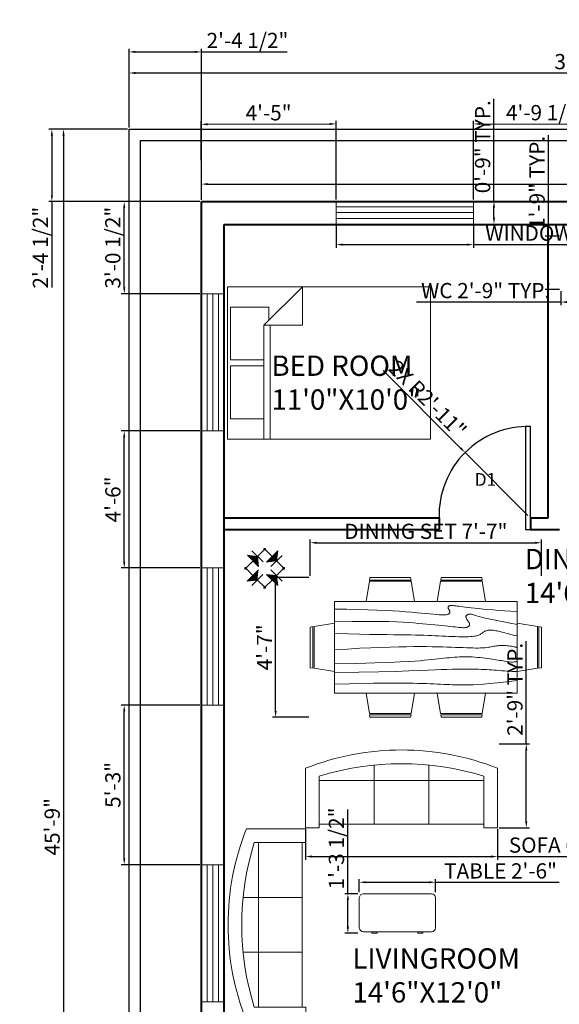
# Model space of a CAD drawing. Units: inches. Extents: x 459864 to 460310, y 324185 to 324787.
# Tile 110 of 112: x 459864 to 460076, y 324400 to 324787. Entities that reach past the tile are written whole.
import ezdxf

# ---------------------------------------------------------------- set-up
doc = ezdxf.new("R2010")
doc.units = ezdxf.units.IN
for name, color, linetype, lineweight in [('A-ANNO-DIMS', 2, 'Continuous', 18), ('A-ANNO-TEXT', 7, 'Continuous', 18), ('A-AREA-IDEN', 7, 'Continuous', 25), ('A-DOOR', 3, 'Continuous', 25), ('A-FURN', 8, 'Continuous', 18), ('A-GLAZ', 4, 'Continuous', 18), ('A-WALL', 7, 'Continuous', 40), ('C-PROP', 7, 'Continuous', 30)]:
    doc.layers.add(name, color=color, linetype=linetype, lineweight=lineweight)
doc.styles.get("Standard").update_dxf_attribs({"font": 'arial.ttf'})
doc.dimstyles.new('ISO-25', dxfattribs={"dimtxt": 6, "dimasz": 2.5, "dimexe": 1.25, "dimexo": 0.625, "dimtad": 1, "dimdec": 1, "dimlunit": 3, "dimtxsty": 'Standard', "dimcen": 2.5, "dimadec": 0, "dimazin": 0, "dimtfac": 1, "dimtdec": 1, "dimtmove": 0, "dimatfit": 3, "dimfxl": 1, "dimarcsym": 0})

# ---------------------------------------------------------------- blocks, each defined once
blk = doc.blocks.new('Window - Wood Frame 36 in. Wide plan')
for p, q in [((0, 6), (0, 0)), ((36, 6), (36, 0)), ((0, 4.5), (36, 4.5)), ((0, 3), (36, 3)), ((0, 1.5), (36, 1.5))]:
    blk.add_line(p, q)
blk = doc.blocks.new('Bed - Queen')
for p, q in [((0, -80.00003), (0, 0)), ((0, 0), (59.99999, 0)), ((59.99999, 0), (59.99999, -80.00003)), ((7.99999, -1.2), (28.79998, -1.2)), ((7.99999, -14.4), (7.99999, -1.2)), ((28.79998, -1.2), (28.79998, -14.4)), ((31.19999, -1.2), (51.99999, -1.2)), ((31.19999, -14.4), (31.19999, -1.2)), ((51.99999, -1.2), (51.99999, -16.4)), ((0, -14.4), (44.8, -14.4)), ((59.99999, -29.6), (44.8, -14.4)), ((44.8, -14.4), (44.8, -29.6)), ((44.8, -16.8), (0, -16.8)), ((51.99999, -16.4), (46.79936, -16.4)), ((44.8, -29.6), (59.99999, -29.6)), ((59.99999, -80.00003), (0, -80.00003))]:
    blk.add_line(p, q)
blk = doc.blocks.new('Dining Set - 36 x 72 in.')
for p, q in [((-22, 27.5), (-22.1562, 26.50042)), ((-22, 27.5), (-6, 27.5)), ((-5.8437, 26.49966), (-6, 27.5)), ((6, 27.5), (5.8438, 26.50042)), ((6, 27.5), (22, 27.5)), ((22.1563, 26.49966), (22, 27.5)), ((-22.2343, 26.00059), (-23.4847, 17.99762)), ((-22.2304, 26), (-5.7608, 26)), ((-5.8416, 26.5), (-22.1534, 26.5)), ((-4.5152, 17.99762), (-5.7655, 25.99926)), ((5.7657, 26.00059), (4.5153, 17.99762)), ((5.7696, 26), (22.2392, 26)), ((22.1584, 26.5), (5.8466, 26.5)), ((23.4848, 17.99762), (22.2345, 25.99926)), ((36, 18), (-36, 18)), ((-36, 18), (-36, -18)), ((36, -18), (36, 18)), ((-45.5, 8), (-44.5004, 8.15617)), ((-45.5, 8), (-45.5, -8)), ((-44.5, -8.15843), (-44.5, 8.15338)), ((-44.0006, 8.23428), (-35.9976, 9.48474)), ((-44, 8.23041), (-44, -8.23915)), ((44.0006, 8.23428), (35.9976, 9.48474)), ((44, 8.23041), (44, -8.23915)), ((44.5, -8.15843), (44.5, 8.15338)), ((45.5, 8), (44.5005, 8.15617)), ((45.5, 8), (45.5, -8)), ((-44.4997, -8.15631), (-45.5, -8)), ((-35.9976, -9.48476), (-43.9993, -8.2345)), ((35.9976, -9.48476), (43.9993, -8.2345)), ((44.4997, -8.15631), (45.5, -8)), ((-36, -18), (36, -18)), ((-22.2343, -26.0006), (-23.4847, -17.99762)), ((-4.5152, -17.99762), (-5.7655, -25.99928)), ((5.7657, -26.0006), (4.5153, -17.99762)), ((23.4848, -17.99762), (22.2345, -25.99928)), ((-22.2304, -26), (-5.7608, -26)), ((-22, -27.5), (-22.1562, -26.50044)), ((-5.8416, -26.5), (-22.1534, -26.5)), ((-5.8437, -26.49967), (-6, -27.5)), ((5.7696, -26), (22.2392, -26)), ((6, -27.5), (5.8438, -26.50044)), ((22.1584, -26.5), (5.8466, -26.5)), ((22.1563, -26.49967), (22, -27.5)), ((-22, -27.5), (-6, -27.5)), ((6, -27.5), (22, -27.5))]:
    blk.add_line(p, q)
for points in [[(-36, 15), (-31.1772, 14.97754), (-26.8079, 14.91406), (-22.8538, 14.81543), (-19.276, 14.6875), (-16.0362, 14.53613), (-13.0957, 14.36718), (-10.4159, 14.18652), (-7.9583, 14), (-5.6904, 13.81315), (-3.6035, 13.63021), (-1.6954, 13.45508), (0.0365, 13.29166), (1.5945, 13.14388), (2.9811, 13.01562), (4.1988, 12.9108), (5.25, 12.83333), (6.1393, 12.78613), (6.8802, 12.76823), (7.4883, 12.77767), (7.9792, 12.8125), (8.3685, 12.87077), (8.6719, 12.95052), (8.9049, 13.0498), (9.0833, 13.16666), (9.2205, 13.29899), (9.3216, 13.44401), (9.3895, 13.59879), (9.4271, 13.76041), (9.4373, 13.92594), (9.4232, 14.09245), (9.3875, 14.257), (9.3333, 14.41666), (9.2638, 14.56917), (9.1836, 14.71484), (9.0975, 14.85465), (9.0104, 14.98958), (8.9272, 15.1206), (8.8529, 15.2487), (8.7922, 15.37483), (8.75, 15.5), (8.7305, 15.62467), (8.7344, 15.74739), (8.7617, 15.86621), (8.8125, 15.97916), (8.8867, 16.08431), (8.9844, 16.17968), (9.1055, 16.26334), (9.25, 16.33333), (9.4189, 16.38802), (9.6172, 16.42708), (9.8506, 16.45052), (10.125, 16.45833), (10.4463, 16.45052), (10.8203, 16.42708), (11.2529, 16.38802), (11.75, 16.33333), (12.3184, 16.26318), (12.9694, 16.17838), (13.7151, 16.07991), (14.5677, 15.96875), (15.5395, 15.84586), (16.6426, 15.71224), (17.8893, 15.56884), (19.2917, 15.41666), (20.859, 15.25667), (22.5879, 15.08984), (24.4721, 14.91715), (26.5052, 14.73958), (28.6809, 14.5581), (30.9929, 14.3737), (33.4347, 14.18733), (36, 14)], [(-36, 10), (-28.9766, 10.14274), (-23.1725, 10.20442), (-18.4241, 10.19775), (-14.5677, 10.13541), (-11.4399, 10.03011), (-8.877, 9.89453), (-6.7154, 9.74137), (-4.7917, 9.58333), (-2.9698, 9.43082), (-1.2246, 9.28515), (0.4415, 9.14534), (2.026, 9.01041), (3.5266, 8.87939), (4.9408, 8.7513), (6.266, 8.62516), (7.5, 8.5), (8.6411, 8.37549), (9.6914, 8.2539), (10.6538, 8.13818), (11.5312, 8.03125), (12.3267, 7.93603), (13.043, 7.85547), (13.6831, 7.79248), (14.25, 7.75), (14.7471, 7.7303), (15.1797, 7.73307), (15.5537, 7.75732), (15.875, 7.80208), (16.1494, 7.86637), (16.3828, 7.94922), (16.5811, 8.04964), (16.75, 8.16666), (16.8944, 8.29915), (17.0143, 8.44531), (17.1089, 8.60319), (17.1771, 8.77083), (17.218, 8.94629), (17.2305, 9.1276), (17.2137, 9.31282), (17.1667, 9.5), (17.0895, 9.6875), (16.987, 9.875), (16.8649, 10.0625), (16.7292, 10.25), (16.5856, 10.4375), (16.4401, 10.625), (16.2985, 10.8125), (16.1667, 11), (16.05, 11.18733), (15.9518, 11.3737), (15.8752, 11.5581), (15.8229, 11.73958), (15.798, 11.91715), (15.8034, 12.08984), (15.842, 12.25667), (15.9167, 12.41666), (16.0295, 12.56836), (16.1784, 12.70833), (16.3605, 12.83268), (16.5729, 12.9375), (16.8127, 13.01888), (17.0768, 13.07291), (17.3625, 13.0957), (17.6667, 13.08333), (17.9894, 13.03312), (18.3418, 12.94726), (18.7382, 12.82918), (19.1927, 12.68229), (19.7195, 12.51001), (20.3327, 12.31575), (21.0465, 12.10294), (21.875, 11.875), (22.8357, 11.63354), (23.959, 11.37304), (25.2786, 11.08618), (26.8282, 10.76562), (28.6414, 10.40405), (30.752, 9.99414), (33.1936, 9.52856), (36, 9)], [(-36, 5.5), (-30.7157, 5.3348), (-26.069, 5.20963), (-21.9946, 5.11767), (-18.4271, 5.05208), (-15.3009, 5.00602), (-12.5508, 4.97265), (-10.1112, 4.94515), (-7.9167, 4.91666), (-5.909, 4.88167), (-4.0586, 4.83984), (-2.3429, 4.79215), (-0.7396, 4.73958), (0.7739, 4.6831), (2.22, 4.6237), (3.6213, 4.56233), (5, 4.5), (6.373, 4.43782), (7.7344, 4.3776), (9.0723, 4.32129), (10.375, 4.27083), (11.6309, 4.22819), (12.8281, 4.19531), (13.9551, 4.17415), (15, 4.16666), (15.954, 4.17448), (16.819, 4.19791), (17.6001, 4.23698), (18.3021, 4.29166), (18.9299, 4.36198), (19.4883, 4.44791), (19.9823, 4.54948), (20.4167, 4.66666), (20.7969, 4.79899), (21.1302, 4.94401), (21.4245, 5.09879), (21.6875, 5.26041), (21.9271, 5.42594), (22.1511, 5.59245), (22.3672, 5.757), (22.5834, 5.91666), (22.8065, 6.06868), (23.0404, 6.21093), (23.2879, 6.34147), (23.5521, 6.45833), (23.8358, 6.55957), (24.142, 6.64323), (24.4735, 6.70735), (24.8334, 6.75), (25.2235, 6.76969), (25.642, 6.76692), (26.0858, 6.74267), (26.5521, 6.69791), (27.0379, 6.63362), (27.5404, 6.55078), (28.0565, 6.45036), (28.5834, 6.33333), (29.1242, 6.19987), (29.7071, 6.04687), (30.3661, 5.87044), (31.1354, 5.66666), (32.0493, 5.43164), (33.142, 5.16146), (34.4475, 4.85221), (36, 4.5)], [(-36, -1), (-30.7915, -0.6591), (-26.0195, -0.38216), (-21.6519, -0.16284), (-17.6563, 0.00521), (-14.0005, 0.12833), (-10.6523, 0.21289), (-7.5796, 0.26522), (-4.75, 0.29166), (-2.134, 0.29793), (0.2878, 0.28711), (2.5317, 0.26163), (4.6146, 0.22396), (6.5529, 0.17651), (8.3633, 0.12174), (10.0623, 0.06209), (11.6667, 0), (13.1899, -0.06201), (14.6341, -0.1211), (15.9982, -0.17432), (17.2813, -0.21875), (18.4823, -0.25147), (19.6003, -0.26953), (20.6343, -0.27002), (21.5834, -0.25), (22.4481, -0.20768), (23.2357, -0.14584), (23.9549, -0.06836), (24.6146, 0.02083), (25.2235, 0.11784), (25.7904, 0.21875), (26.3241, 0.31966), (26.8334, 0.41666), (27.3265, 0.50618), (27.8099, 0.58593), (28.2894, 0.65397), (28.7709, 0.70833), (29.2601, 0.74707), (29.763, 0.76823), (30.2855, 0.76985), (30.8334, 0.75), (31.4088, 0.70784), (31.9994, 0.64713), (32.589, 0.57275), (33.1615, 0.48958), (33.7008, 0.4025), (34.1908, 0.3164), (34.6153, 0.23616), (34.9584, 0.16666), (35.2099, 0.11165), (35.3848, 0.07031), (35.504, 0.04069), (35.5886, 0.02083), (35.6594, 0.00879), (35.7377, 0.0026), (35.8442, 0.00032), (36, 0)], [(-36, -6.5), (-27.1843, -6.31267), (-20.084, -6.1263), (-14.469, -5.9419), (-10.1094, -5.76042), (-6.7752, -5.58285), (-4.2363, -5.41016), (-2.2629, -5.24333), (-0.625, -5.08334), (0.8708, -4.93099), (2.2715, -4.78646), (3.5872, -4.64974), (4.8281, -4.52084), (6.0046, -4.39974), (7.127, -4.28646), (8.2053, -4.18099), (9.25, -4.08334), (10.2705, -3.99382), (11.2734, -3.91407), (12.2647, -3.84603), (13.25, -3.79167), (14.2354, -3.75293), (15.2266, -3.73177), (16.2295, -3.73015), (17.25, -3.75), (18.2912, -3.79248), (19.3451, -3.85547), (20.4009, -3.93604), (21.4479, -4.03125), (22.4754, -4.13819), (23.4727, -4.25391), (24.4289, -4.37549), (25.3334, -4.5), (26.1785, -4.62492), (26.9694, -4.74935), (27.7145, -4.87281), (28.4219, -4.99479), (29.1, -5.11483), (29.7572, -5.23242), (30.4016, -5.34709), (31.0417, -5.45834), (31.6837, -5.56437), (32.3262, -5.65821), (32.9658, -5.73153), (33.599, -5.77604), (34.2224, -5.78345), (34.8327, -5.74545), (35.4264, -5.65373), (36, -5.5)], [(-36, -10), (-26.4022, -9.81299), (-18.4675, -9.62891), (-11.9839, -9.45069), (-6.7396, -9.28125), (-2.5226, -9.12354), (0.8789, -8.98047), (3.6769, -8.85498), (6.0833, -8.75), (8.2767, -8.66765), (10.3021, -8.60677), (12.1712, -8.56543), (13.8958, -8.54167), (15.4876, -8.53353), (16.9583, -8.53907), (18.3197, -8.55632), (19.5834, -8.58334), (20.7616, -8.61841), (21.8685, -8.66081), (22.9188, -8.71004), (23.9271, -8.76563), (24.9081, -8.82707), (25.8763, -8.89388), (26.8465, -8.96558), (27.8334, -9.04167), (28.8474, -9.12118), (29.8828, -9.20117), (30.93, -9.27824), (31.9792, -9.34896), (33.0205, -9.40991), (34.0443, -9.45768), (35.0407, -9.48885), (36, -9.5)], [(-36, -14.5), (-30.0881, -14.33513), (-25.0332, -14.21224), (-20.7312, -14.12647), (-17.0781, -14.07292), (-13.97, -14.04671), (-11.3027, -14.04297), (-8.9724, -14.05681), (-6.875, -14.08334), (-4.9224, -14.11833), (-3.0905, -14.16016), (-1.3709, -14.20785), (0.2448, -14.26042), (1.7647, -14.3169), (3.1973, -14.3763), (4.5507, -14.43767), (5.8333, -14.5), (7.0554, -14.5621), (8.235, -14.62175), (9.3922, -14.67652), (10.5469, -14.72396), (11.7192, -14.76164), (12.929, -14.78711), (14.1965, -14.79794), (15.5417, -14.79167), (16.9933, -14.76424), (18.6152, -14.70508), (20.4804, -14.60197), (22.6615, -14.44271), (25.2312, -14.21509), (28.2624, -13.9069), (31.8277, -13.50594), (36, -13)]]:
    blk.add_lwpolyline(points)
blk = doc.blocks.new('Full Wave Bridge')
for p, q in [((0.026823, 0.204407), (0.185922, 0.186729)), ((0.2036, 0.02763), (0.026823, 0.204407)), ((0.274311, 0.098341), (0.097534, 0.275118)), ((0.185922, 0.186729), (0.3, 0.3)), ((0.185922, 0.186729), (0.2036, 0.02763)), ((0.415786, 0.185084), (0.3, 0.3)), ((0.327398, 0.096696), (0.504174, 0.273472)), ((0.398109, 0.025985), (0.574885, 0.202762)), ((0.504174, 0.273472), (0.486497, 0.114373)), ((0.115212, 0.116019), (0, 0)), ((0.113504, -0.114373), (0, 0)), ((0.115212, 0.116019), (0.122283, 0.12309)), ((0.486497, 0.114373), (0.327398, 0.096696)), ((0.486497, 0.114373), (0.6, 0)), ((0.486497, -0.114373), (0.6, 0)), ((0.025116, -0.202762), (0.201892, -0.025985)), ((0.095826, -0.273472), (0.272603, -0.096695)), ((0.113504, -0.114373), (0.120575, -0.121444)), ((0.120575, -0.121444), (0.127646, -0.128515)), ((0.127646, -0.128515), (0.134717, -0.135586)), ((0.134717, -0.135586), (0.141788, -0.142657)), ((0.141788, -0.142657), (0.15593, -0.1568)), ((0.155993, -0.148218), (0.148824, -0.154349)), ((0.327398, -0.096695), (0.486497, -0.114373)), ((0.504174, -0.273472), (0.327398, -0.096695)), ((0.574885, -0.202762), (0.398108, -0.025985)), ((0.486497, -0.114373), (0.504174, -0.273472)), ((0.184215, -0.185084), (0.025116, -0.202762)), ((0.184215, -0.185084), (0.3, -0.3)), ((0.415786, -0.185084), (0.3, -0.3)), ((0.415786, -0.185084), (0.422857, -0.178013))]:
    blk.add_line(p, q)
for points in [[(0.2875, 0.2875), (0.2875, 0.3125), (0.3125, 0.3125), (0.3125, 0.2875)], [(-0.0125, -0.0125), (-0.0125, 0.0125), (0.012501, 0.0125), (0.012501, -0.0125)], [(0.5875, -0.0125), (0.5875, 0.0125), (0.6125, 0.0125), (0.6125, -0.0125)], [(0.2875, -0.3125), (0.2875, -0.2875), (0.3125, -0.2875), (0.3125, -0.3125)]]:
    blk.add_lwpolyline(points, close=True)
for points in [[(0.3125, 0.2875), (0.3125, 0.3125), (0.2875, 0.3125)], [(0.2875, 0.3125), (0.2875, 0.2875), (0.3125, 0.2875)], [(0.2036, 0.02763), (0.185922, 0.186729), (0.026823, 0.204407)], [(0.327398, 0.096696), (0.486497, 0.114373), (0.504174, 0.273472)], [(0.012501, -0.0125), (0.012501, 0.0125), (-0.0125, 0.0125)], [(-0.0125, 0.0125), (-0.0125, -0.0125), (0.012501, -0.0125)], [(0.6125, -0.0125), (0.6125, 0.0125), (0.5875, 0.0125)], [(0.5875, 0.0125), (0.5875, -0.0125), (0.6125, -0.0125)], [(0.025116, -0.202762), (0.184215, -0.185084), (0.201892, -0.025985)], [(0.327398, -0.096695), (0.486497, -0.114373), (0.504174, -0.273472)], [(0.3125, -0.3125), (0.3125, -0.2875), (0.2875, -0.2875)], [(0.2875, -0.2875), (0.2875, -0.3125), (0.3125, -0.3125)]]:
    blk.add_solid(points)
blk = doc.blocks.new('Sofa - Roundback 7 ft.')
for p, q in [((-12.00002, -32.4421), (-12.00003, -6.5971)), ((11.99997, -32.4421), (11.99998, -6.5971)), ((-36.000027, -34), (-36.000027, -11.4696)), ((35.99998, -34), (35.99998, -11.4696)), ((-35.999844, -13.3819), (35.9998, -13.3819)), ((-36.000027, -32.4421), (35.99998, -32.4421))]:
    blk.add_line(p, q)
for points in [[(-36.000027, -34), (-42.000027, -34), (-42.000027, -8)], [(41.99998, -8), (41.99998, -34), (35.99998, -34)]]:
    blk.add_lwpolyline(points)
for centre, radius, start, end in [((0, -114.25), 114.25, 68.43141, 111.5686), ((-0.00001, -127.1968), 121.1968, 72.72033, 107.2797)]:
    blk.add_arc(centre, radius, start, end)
blk = doc.blocks.new('Desk - 30 x 60 in.')
for p, q in [((-26.999995, 0), (26.999995, 0)), ((-29.999995, -27), (-29.999995, -3)), ((29.999995, -3), (29.999995, -27)), ((26.999995, -30), (-26.999995, -30)), ((-20.000005, -30), (-20.000005, -31)), ((-16.000005, -31), (-16.000005, -30)), ((15.999995, -31), (15.999995, -30)), ((19.999995, -30), (19.999995, -31)), ((-20.000005, -31), (-16.000005, -31)), ((19.999995, -31), (15.999995, -31))]:
    blk.add_line(p, q)
for centre, start, end in [((-26.499995, -3.5), 98.1301, 171.8699), ((26.499995, -3.5), 8.130102, 81.8699), ((-26.499995, -26.5), 188.1301, 261.8699), ((26.499995, -26.5), 278.1301, 351.8699)]:
    blk.add_arc(centre, 3.535534, start, end)
blk = doc.blocks.new('*D19')
at = {"layer": 'A-ANNO-DIMS', "color": 0, "lineweight": -2, "transparency": 16777216}
for p, q in [((459935.11, 324716.11), (459935.11, 324723.62)), ((460247.11, 324716.11), (460247.11, 324723.62)), ((459937.61, 324722.37), (460244.61, 324722.37))]:
    blk.add_line(p, q, dxfattribs=at)
at = {"layer": 'A-ANNO-DIMS', "color": 0, "transparency": 16777216}
for points in [[(459937.61, 324722.79), (459937.61, 324721.96), (459935.11, 324722.37)], [(460244.61, 324722.79), (460244.61, 324721.96), (460247.11, 324722.37)]]:
    blk.add_solid(points, dxfattribs=at)
at = {"layer": 'Defpoints', "color": 0, "transparency": 16777216}
for p in [(460247.11, 324722.37), (459935.11, 324715.48), (460247.11, 324715.48)]:
    blk.add_point(p, dxfattribs=at)
at = {"layer": 'A-ANNO-DIMS', "color": 0, "transparency": 16777216, "insert": (460091.11, 324726.06), "char_height": 6, "attachment_point": 5}
blk.add_mtext("26'", dxfattribs=at)
blk = doc.blocks.new('*D20')
at = {"layer": 'A-ANNO-DIMS', "color": 0, "lineweight": -2, "transparency": 16777216}
for p, q in [((459906.61, 324744.61), (459906.61, 324767.34)), ((459909.11, 324766.09), (460268.61, 324766.09)), ((460271.11, 324744.61), (460271.11, 324767.34))]:
    blk.add_line(p, q, dxfattribs=at)
at = {"layer": 'A-ANNO-DIMS', "color": 0, "transparency": 16777216}
for points in [[(459909.11, 324766.5), (459909.11, 324765.67), (459906.61, 324766.09)], [(460268.61, 324766.5), (460268.61, 324765.67), (460271.11, 324766.09)]]:
    blk.add_solid(points, dxfattribs=at)
at = {"layer": 'Defpoints', "color": 0, "transparency": 16777216}
for p in [(460271.11, 324766.09), (459906.61, 324743.98), (460271.11, 324743.98)]:
    blk.add_point(p, dxfattribs=at)
at = {"layer": 'A-ANNO-DIMS', "color": 0, "transparency": 16777216, "insert": (460088.86, 324769.78), "char_height": 6, "attachment_point": 5}
blk.add_mtext('30\'-4.5"', dxfattribs=at)
blk = doc.blocks.new('*D22')
at = {"layer": 'A-ANNO-DIMS', "color": 0, "lineweight": -2, "transparency": 16777216}
for p, q in [((459905.99, 324743.98), (459879.56, 324743.98)), ((459880.81, 324741.48), (459880.81, 324197.48)), ((459905.99, 324194.98), (459879.56, 324194.98))]:
    blk.add_line(p, q, dxfattribs=at)
at = {"layer": 'A-ANNO-DIMS', "color": 0, "transparency": 16777216}
for points in [[(459880.39, 324741.48), (459881.22, 324741.48), (459880.81, 324743.98)], [(459880.39, 324197.48), (459881.22, 324197.48), (459880.81, 324194.98)]]:
    blk.add_solid(points, dxfattribs=at)
at = {"layer": 'Defpoints', "color": 0, "transparency": 16777216}
for p in [(459906.61, 324743.98), (459880.81, 324194.98), (459906.61, 324194.98)]:
    blk.add_point(p, dxfattribs=at)
at = {"layer": 'A-ANNO-DIMS', "color": 0, "transparency": 16777216, "insert": (459877.12, 324469.48), "char_height": 6, "attachment_point": 5, "rotation": 90}
blk.add_mtext('45\'-9"', dxfattribs=at)
blk = doc.blocks.new('DOOR-SWING-36IN')
for p, q in [((40.5, 2), (0, 2)), ((0, 2), (0, 0)), ((40.5, 0), (40.5, 2)), ((4.5, 0), (40.5, 0))]:
    blk.add_line(p, q)
blk.add_arc((5.5, 1), 35.01, 358.3634, 91.6366)
blk = doc.blocks.new('*D24')
at = {"layer": 'A-ANNO-DIMS', "color": 0, "lineweight": -2, "transparency": 16777216}
for p, q in [((459988.23, 324706.02), (459988.23, 324697.29)), ((460042.23, 324706.02), (460042.23, 324697.29)), ((459990.73, 324698.54), (460039.73, 324698.54)), ((460042.23, 324698.54), (460121.9, 324698.54))]:
    blk.add_line(p, q, dxfattribs=at)
at = {"layer": 'A-ANNO-DIMS', "color": 0, "transparency": 16777216}
for points in [[(459990.73, 324698.96), (459990.73, 324698.13), (459988.23, 324698.54)], [(460039.73, 324698.96), (460039.73, 324698.13), (460042.23, 324698.54)]]:
    blk.add_solid(points, dxfattribs=at)
at = {"layer": 'Defpoints', "color": 0, "transparency": 16777216}
for p in [(459988.23, 324706.64), (460042.23, 324706.64), (460042.23, 324698.54)]:
    blk.add_point(p, dxfattribs=at)
at = {"layer": 'A-ANNO-DIMS', "color": 0, "transparency": 16777216, "insert": (460083.32, 324702.27), "char_height": 6, "attachment_point": 5}
blk.add_mtext('WINDOW 4\'-6" TYP.', dxfattribs=at)
blk = doc.blocks.new('*D25')
at = {"layer": 'A-ANNO-DIMS', "color": 0, "lineweight": -2, "transparency": 16777216}
for p, q in [((460050.33, 324715.64), (460050.33, 324755.97)), ((460042.85, 324715.64), (460051.58, 324715.64)), ((460050.33, 324709.14), (460050.33, 324713.14)), ((460042.85, 324706.64), (460051.58, 324706.64))]:
    blk.add_line(p, q, dxfattribs=at)
at = {"layer": 'A-ANNO-DIMS', "color": 0, "transparency": 16777216}
for points in [[(460049.91, 324713.14), (460050.75, 324713.14), (460050.33, 324715.64)], [(460049.91, 324709.14), (460050.75, 324709.14), (460050.33, 324706.64)]]:
    blk.add_solid(points, dxfattribs=at)
at = {"layer": 'Defpoints', "color": 0, "transparency": 16777216}
for p in [(460042.23, 324715.64), (460050.33, 324715.64), (460042.23, 324706.64)]:
    blk.add_point(p, dxfattribs=at)
at = {"layer": 'A-ANNO-DIMS', "color": 0, "transparency": 16777216, "insert": (460046.64, 324737.05), "char_height": 6, "attachment_point": 5, "rotation": 90}
blk.add_mtext('0\'-9" TYP.', dxfattribs=at)
blk = doc.blocks.new('*D30')
at = {"layer": 'A-ANNO-DIMS', "color": 0, "lineweight": -2, "transparency": 16777216}
for p, q in [((460076.72, 324680.27), (460076.72, 324674.69)), ((460109.77, 324680.27), (460109.77, 324674.69)), ((460076.72, 324675.94), (460019.86, 324675.94)), ((460107.27, 324675.94), (460079.22, 324675.94))]:
    blk.add_line(p, q, dxfattribs=at)
at = {"layer": 'A-ANNO-DIMS', "color": 0, "transparency": 16777216}
for points in [[(460079.22, 324676.36), (460079.22, 324675.52), (460076.72, 324675.94)], [(460107.27, 324676.36), (460107.27, 324675.52), (460109.77, 324675.94)]]:
    blk.add_solid(points, dxfattribs=at)
at = {"layer": 'Defpoints', "color": 0, "transparency": 16777216}
for p in [(460076.72, 324680.9), (460109.77, 324680.9), (460076.72, 324675.94)]:
    blk.add_point(p, dxfattribs=at)
at = {"layer": 'A-ANNO-DIMS', "color": 0, "transparency": 16777216, "insert": (460047.04, 324679.67), "char_height": 6, "attachment_point": 5}
blk.add_mtext('WC 2\'-9" TYP.', dxfattribs=at)
blk = doc.blocks.new('*D31')
at = {"layer": 'A-ANNO-DIMS', "color": 0, "lineweight": -2, "transparency": 16777216}
for p, q in [((460071.76, 324701.9), (460071.76, 324741.66)), ((460076.09, 324701.9), (460070.51, 324701.9)), ((460071.76, 324683.4), (460071.76, 324699.4)), ((460076.09, 324680.9), (460070.51, 324680.9))]:
    blk.add_line(p, q, dxfattribs=at)
at = {"layer": 'A-ANNO-DIMS', "color": 0, "transparency": 16777216}
for points in [[(460071.35, 324699.4), (460072.18, 324699.4), (460071.76, 324701.9)], [(460071.35, 324683.4), (460072.18, 324683.4), (460071.76, 324680.9)]]:
    blk.add_solid(points, dxfattribs=at)
at = {"layer": 'Defpoints', "color": 0, "transparency": 16777216}
for p in [(460071.76, 324701.9), (460076.72, 324701.9), (460076.72, 324680.9)]:
    blk.add_point(p, dxfattribs=at)
at = {"layer": 'A-ANNO-DIMS', "color": 0, "transparency": 16777216, "insert": (460068.07, 324723.03), "char_height": 6, "attachment_point": 5, "rotation": 90}
blk.add_mtext('1\'-9" TYP.', dxfattribs=at)
blk = doc.blocks.new('*D32')
at = {"layer": 'A-ANNO-DIMS', "color": 0, "lineweight": -2, "transparency": 16777216}
for p, q in [((459976.12, 324468.46), (459976.12, 324456.5)), ((460051.72, 324468.46), (460051.72, 324456.5)), ((459978.62, 324457.75), (460049.22, 324457.75)), ((460051.72, 324457.75), (460131.14, 324457.75))]:
    blk.add_line(p, q, dxfattribs=at)
at = {"layer": 'A-ANNO-DIMS', "color": 0, "transparency": 16777216}
for points in [[(459978.62, 324458.17), (459978.62, 324457.33), (459976.12, 324457.75)], [(460049.22, 324458.17), (460049.22, 324457.33), (460051.72, 324457.75)]]:
    blk.add_solid(points, dxfattribs=at)
at = {"layer": 'Defpoints', "color": 0, "transparency": 16777216}
for p in [(459976.12, 324469.09), (460051.72, 324469.09), (460051.72, 324457.75)]:
    blk.add_point(p, dxfattribs=at)
at = {"layer": 'A-ANNO-DIMS', "color": 0, "transparency": 16777216, "insert": (460092.68, 324461.48), "char_height": 6, "attachment_point": 5}
blk.add_mtext('SOFA 6\'-3 1/2" TYP.', dxfattribs=at)
blk = doc.blocks.new('*D33')
at = {"layer": 'A-ANNO-DIMS', "color": 0, "lineweight": -2, "transparency": 16777216}
for p, q in [((460063.06, 324502.09), (460063.06, 324542.51)), ((460052.34, 324502.09), (460064.31, 324502.09)), ((460063.06, 324471.59), (460063.06, 324499.59)), ((460052.34, 324469.09), (460064.31, 324469.09))]:
    blk.add_line(p, q, dxfattribs=at)
at = {"layer": 'A-ANNO-DIMS', "color": 0, "transparency": 16777216}
for points in [[(460062.64, 324499.59), (460063.47, 324499.59), (460063.06, 324502.09)], [(460062.64, 324471.59), (460063.47, 324471.59), (460063.06, 324469.09)]]:
    blk.add_solid(points, dxfattribs=at)
at = {"layer": 'Defpoints', "color": 0, "transparency": 16777216}
for p in [(460051.72, 324502.09), (460063.06, 324502.09), (460051.72, 324469.09)]:
    blk.add_point(p, dxfattribs=at)
at = {"layer": 'A-ANNO-DIMS', "color": 0, "transparency": 16777216, "insert": (460059.37, 324523.55), "char_height": 6, "attachment_point": 5, "rotation": 90}
blk.add_mtext('2\'-9" TYP.', dxfattribs=at)
blk = doc.blocks.new('*D40')
at = {"layer": 'A-ANNO-DIMS', "color": 0, "lineweight": -2, "transparency": 16777216}
for p, q in [((459978, 324568.2), (459978, 324582.47)), ((459980.5, 324581.22), (460066.5, 324581.22)), ((460069, 324568.2), (460069, 324582.47))]:
    blk.add_line(p, q, dxfattribs=at)
at = {"layer": 'A-ANNO-DIMS', "color": 0, "transparency": 16777216}
for points in [[(459980.5, 324581.64), (459980.5, 324580.81), (459978, 324581.22)], [(460066.5, 324581.64), (460066.5, 324580.81), (460069, 324581.22)]]:
    blk.add_solid(points, dxfattribs=at)
at = {"layer": 'Defpoints', "color": 0, "transparency": 16777216}
for p in [(460069, 324581.22), (459978, 324567.57), (460069, 324567.57)]:
    blk.add_point(p, dxfattribs=at)
at = {"layer": 'A-ANNO-DIMS', "color": 0, "transparency": 16777216, "insert": (460023.5, 324584.95), "char_height": 6, "attachment_point": 5}
blk.add_mtext('DINING SET 7\'-7"', dxfattribs=at)
blk = doc.blocks.new('*D41')
at = {"layer": 'A-ANNO-DIMS', "color": 0, "lineweight": -2, "transparency": 16777216}
for p, q in [((459977.37, 324567.57), (459963.1, 324567.57)), ((459964.35, 324515.07), (459964.35, 324565.07)), ((459977.37, 324512.57), (459963.1, 324512.57))]:
    blk.add_line(p, q, dxfattribs=at)
at = {"layer": 'A-ANNO-DIMS', "color": 0, "transparency": 16777216}
for points in [[(459963.93, 324565.07), (459964.76, 324565.07), (459964.35, 324567.57)], [(459963.93, 324515.07), (459964.76, 324515.07), (459964.35, 324512.57)]]:
    blk.add_solid(points, dxfattribs=at)
at = {"layer": 'Defpoints', "color": 0, "transparency": 16777216}
for p in [(459964.35, 324567.57), (459978, 324567.57), (459978, 324512.57)]:
    blk.add_point(p, dxfattribs=at)
at = {"layer": 'A-ANNO-DIMS', "color": 0, "transparency": 16777216, "insert": (459960.72, 324540.07), "char_height": 6, "attachment_point": 5, "rotation": 90}
blk.add_mtext('4\'-7"', dxfattribs=at)
blk = doc.blocks.new('*D44')
at = {"layer": 'A-ANNO-DIMS', "color": 0, "lineweight": -2, "transparency": 16777216}
for p, q in [((459997.29, 324443.76), (459997.29, 324448.88)), ((460027.29, 324443.76), (460027.29, 324448.88)), ((459999.79, 324447.63), (460024.79, 324447.63)), ((460027.29, 324447.63), (460076.02, 324447.63))]:
    blk.add_line(p, q, dxfattribs=at)
at = {"layer": 'A-ANNO-DIMS', "color": 0, "transparency": 16777216}
for points in [[(459999.79, 324448.05), (459999.79, 324447.22), (459997.29, 324447.63)], [(460024.79, 324448.05), (460024.79, 324447.22), (460027.29, 324447.63)]]:
    blk.add_solid(points, dxfattribs=at)
at = {"layer": 'Defpoints', "color": 0, "transparency": 16777216}
for p in [(460027.29, 324447.63), (459997.29, 324443.13), (460027.29, 324443.13)]:
    blk.add_point(p, dxfattribs=at)
at = {"layer": 'A-ANNO-DIMS', "color": 0, "transparency": 16777216, "insert": (460052.91, 324451.32), "char_height": 6, "attachment_point": 5}
blk.add_mtext('TABLE 2\'-6"', dxfattribs=at)
blk = doc.blocks.new('*D45')
at = {"layer": 'A-ANNO-DIMS', "color": 0, "lineweight": -2, "transparency": 16777216}
for p, q in [((459992.79, 324443.13), (459992.79, 324476.25)), ((459996.66, 324443.13), (459991.54, 324443.13)), ((459992.79, 324430.13), (459992.79, 324440.63)), ((459996.66, 324427.63), (459991.54, 324427.63))]:
    blk.add_line(p, q, dxfattribs=at)
at = {"layer": 'A-ANNO-DIMS', "color": 0, "transparency": 16777216}
for points in [[(459992.37, 324440.63), (459993.21, 324440.63), (459992.79, 324443.13)], [(459992.37, 324430.13), (459993.21, 324430.13), (459992.79, 324427.63)]]:
    blk.add_solid(points, dxfattribs=at)
at = {"layer": 'Defpoints', "color": 0, "transparency": 16777216}
for p in [(459992.79, 324443.13), (459997.29, 324443.13), (459997.29, 324427.63)]:
    blk.add_point(p, dxfattribs=at)
at = {"layer": 'A-ANNO-DIMS', "color": 0, "transparency": 16777216, "insert": (459989.06, 324460.94), "char_height": 6, "attachment_point": 5, "rotation": 90}
blk.add_mtext('1\'-3 1/2"', dxfattribs=at)
blk = doc.blocks.new('*D54')
at = {"layer": 'A-ANNO-DIMS', "color": 0, "lineweight": -2, "transparency": 16777216}
for p, q in [((459906.61, 324744.61), (459906.61, 324775.63)), ((459909.11, 324774.38), (459932.61, 324774.38)), ((459935.11, 324716.11), (459935.11, 324775.63)), ((459935.11, 324774.38), (459968.9, 324774.38))]:
    blk.add_line(p, q, dxfattribs=at)
at = {"layer": 'A-ANNO-DIMS', "color": 0, "transparency": 16777216}
for points in [[(459909.11, 324774.8), (459909.11, 324773.97), (459906.61, 324774.38)], [(459932.61, 324774.8), (459932.61, 324773.97), (459935.11, 324774.38)]]:
    blk.add_solid(points, dxfattribs=at)
at = {"layer": 'Defpoints', "color": 0, "transparency": 16777216}
for p in [(459935.11, 324774.38), (459906.61, 324743.98), (459935.11, 324715.48)]:
    blk.add_point(p, dxfattribs=at)
at = {"layer": 'A-ANNO-DIMS', "color": 0, "transparency": 16777216, "insert": (459953.26, 324778.11), "char_height": 6, "attachment_point": 5}
blk.add_mtext('2\'-4 1/2"', dxfattribs=at)
blk = doc.blocks.new('*D55')
at = {"layer": 'A-ANNO-DIMS', "color": 0, "lineweight": -2, "transparency": 16777216}
for p, q in [((459905.99, 324743.98), (459874.96, 324743.98)), ((459876.21, 324741.48), (459876.21, 324717.98)), ((459934.49, 324715.48), (459874.96, 324715.48)), ((459876.21, 324715.48), (459876.21, 324681.7))]:
    blk.add_line(p, q, dxfattribs=at)
at = {"layer": 'A-ANNO-DIMS', "color": 0, "transparency": 16777216}
for points in [[(459875.8, 324741.48), (459876.63, 324741.48), (459876.21, 324743.98)], [(459875.8, 324717.98), (459876.63, 324717.98), (459876.21, 324715.48)]]:
    blk.add_solid(points, dxfattribs=at)
at = {"layer": 'Defpoints', "color": 0, "transparency": 16777216}
for p in [(459906.61, 324743.98), (459876.21, 324715.48), (459935.11, 324715.48)]:
    blk.add_point(p, dxfattribs=at)
at = {"layer": 'A-ANNO-DIMS', "color": 0, "transparency": 16777216, "insert": (459872.49, 324697.34), "char_height": 6, "attachment_point": 5, "rotation": 90}
blk.add_mtext('2\'-4 1/2"', dxfattribs=at)
blk = doc.blocks.new('*D56')
at = {"layer": 'A-ANNO-DIMS', "color": 0, "lineweight": -2, "transparency": 16777216}
for p, q in [((459935.11, 324716.11), (459935.02, 324747.13)), ((459988.23, 324716.27), (459988.13, 324747.29)), ((459937.52, 324745.89), (459985.64, 324746.04))]:
    blk.add_line(p, q, dxfattribs=at)
at = {"layer": 'A-ANNO-DIMS', "color": 0, "transparency": 16777216}
for points in [[(459937.52, 324746.31), (459937.52, 324745.47), (459935.02, 324745.88)], [(459985.64, 324746.45), (459985.64, 324745.62), (459988.14, 324746.04)]]:
    blk.add_solid(points, dxfattribs=at)
at = {"layer": 'Defpoints', "color": 0, "transparency": 16777216}
for p in [(459988.14, 324746.04), (459935.11, 324715.48), (459988.23, 324715.64)]:
    blk.add_point(p, dxfattribs=at)
at = {"layer": 'A-ANNO-DIMS', "color": 0, "transparency": 16777216, "insert": (459961.57, 324749.64), "char_height": 6, "attachment_point": 5, "rotation": 0.1723}
blk.add_mtext('4\'-5"', dxfattribs=at)
blk = doc.blocks.new('*D57')
at = {"layer": 'A-ANNO-DIMS', "color": 0, "lineweight": -2, "transparency": 16777216}
for p, q in [((460042.23, 324716.27), (460042.32, 324747.29)), ((460099.91, 324716.11), (460100, 324747.13)), ((460044.81, 324746.04), (460097.5, 324745.89))]:
    blk.add_line(p, q, dxfattribs=at)
at = {"layer": 'A-ANNO-DIMS', "color": 0, "transparency": 16777216}
for points in [[(460044.81, 324746.45), (460044.81, 324745.62), (460042.31, 324746.04)], [(460097.5, 324746.31), (460097.49, 324745.47), (460100, 324745.88)]]:
    blk.add_solid(points, dxfattribs=at)
at = {"layer": 'Defpoints', "color": 0, "transparency": 16777216}
for p in [(460100, 324745.88), (460042.23, 324715.64), (460099.91, 324715.48)]:
    blk.add_point(p, dxfattribs=at)
at = {"layer": 'A-ANNO-DIMS', "color": 0, "transparency": 16777216, "insert": (460071.16, 324749.69), "char_height": 6, "attachment_point": 5, "rotation": 359.8413}
blk.add_mtext('4\'-9 1/2"', dxfattribs=at)
blk = doc.blocks.new('*D59')
at = {"layer": 'A-ANNO-DIMS', "color": 0, "lineweight": -2, "transparency": 16777216}
for p, q in [((459934.49, 324715.48), (459903.46, 324715.48)), ((459904.71, 324681.71), (459904.71, 324712.98)), ((459934.49, 324679.21), (459903.46, 324679.21))]:
    blk.add_line(p, q, dxfattribs=at)
at = {"layer": 'A-ANNO-DIMS', "color": 0, "transparency": 16777216}
for points in [[(459904.3, 324712.98), (459905.13, 324712.98), (459904.71, 324715.48)], [(459904.3, 324681.71), (459905.13, 324681.71), (459904.71, 324679.21)]]:
    blk.add_solid(points, dxfattribs=at)
at = {"layer": 'Defpoints', "color": 0, "transparency": 16777216}
for p in [(459904.71, 324715.48), (459935.11, 324715.48), (459935.11, 324679.21)]:
    blk.add_point(p, dxfattribs=at)
at = {"layer": 'A-ANNO-DIMS', "color": 0, "transparency": 16777216, "insert": (459900.99, 324697.34), "char_height": 6, "attachment_point": 5, "rotation": 90}
blk.add_mtext('3\'-0 1/2"', dxfattribs=at)
blk = doc.blocks.new('*D60')
at = {"layer": 'A-ANNO-DIMS', "color": 0, "lineweight": -2, "transparency": 16777216}
for p, q in [((459934.49, 324625.21), (459903.46, 324625.21)), ((459904.71, 324573.83), (459904.71, 324622.71)), ((459934.49, 324571.33), (459903.46, 324571.33))]:
    blk.add_line(p, q, dxfattribs=at)
at = {"layer": 'A-ANNO-DIMS', "color": 0, "transparency": 16777216}
for points in [[(459904.3, 324622.71), (459905.13, 324622.71), (459904.71, 324625.21)], [(459904.3, 324573.83), (459905.13, 324573.83), (459904.71, 324571.33)]]:
    blk.add_solid(points, dxfattribs=at)
at = {"layer": 'Defpoints', "color": 0, "transparency": 16777216}
for p in [(459904.71, 324625.21), (459935.11, 324625.21), (459935.11, 324571.33)]:
    blk.add_point(p, dxfattribs=at)
at = {"layer": 'A-ANNO-DIMS', "color": 0, "transparency": 16777216, "insert": (459901.03, 324598.27), "char_height": 6, "attachment_point": 5, "rotation": 90}
blk.add_mtext('4\'-6"', dxfattribs=at)
blk = doc.blocks.new('*D61')
at = {"layer": 'A-ANNO-DIMS', "color": 0, "lineweight": -2, "transparency": 16777216}
for p, q in [((459934.49, 324517.33), (459903.46, 324517.33)), ((459904.71, 324457.05), (459904.71, 324514.83)), ((459934.49, 324454.55), (459903.46, 324454.55))]:
    blk.add_line(p, q, dxfattribs=at)
at = {"layer": 'A-ANNO-DIMS', "color": 0, "transparency": 16777216}
for points in [[(459904.3, 324514.83), (459905.13, 324514.83), (459904.71, 324517.33)], [(459904.3, 324457.05), (459905.13, 324457.05), (459904.71, 324454.55)]]:
    blk.add_solid(points, dxfattribs=at)
at = {"layer": 'Defpoints', "color": 0, "transparency": 16777216}
for p in [(459904.71, 324517.33), (459935.11, 324517.33), (459935.11, 324454.55)]:
    blk.add_point(p, dxfattribs=at)
at = {"layer": 'A-ANNO-DIMS', "color": 0, "transparency": 16777216, "insert": (459901.02, 324485.94), "char_height": 6, "attachment_point": 5, "rotation": 90}
blk.add_mtext('5\'-3"', dxfattribs=at)
blk = doc.blocks.new('*D71')
at = {"layer": 'A-ANNO-DIMS', "color": 0, "lineweight": -2, "transparency": 16777216}
for p, q in [((460006.71, 324648.98), (460037.19, 324618.51)), ((460063.71, 324591.98), (460038.95, 324616.74))]:
    blk.add_line(p, q, dxfattribs=at)
at = {"layer": 'A-ANNO-DIMS', "color": 0, "transparency": 16777216}
blk.add_solid([(460037.48, 324618.8), (460036.89, 324618.22), (460038.95, 324616.74)], dxfattribs=at)
at = {"layer": 'Defpoints', "color": 0, "transparency": 16777216}
for p in [(460038.95, 324616.74), (460063.71, 324591.98)]:
    blk.add_point(p, dxfattribs=at)
at = {"layer": 'A-ANNO-DIMS', "color": 0, "transparency": 16777216, "insert": (460023.64, 324637.2), "char_height": 6, "attachment_point": 5, "rotation": 314.9998}
blk.add_mtext('2X R2\'-11"', dxfattribs=at)

msp = doc.modelspace()

# ---------------------------------------------------------------- linework, layer by layer
at = {"layer": 'A-WALL'}
for p, q in [((459935.11, 324715.48), (460247.11, 324715.48)), ((459935.11, 324283.48), (459935.11, 324715.48)), ((459944.11, 324706.48), (460238.11, 324706.48)), ((459944.11, 324283.48), (459944.11, 324706.48)), ((460071.61, 324590.98), (460071.61, 324706.48)), ((459944.11, 324590.98), (460028.71, 324590.98)), ((460028.71, 324590.98), (460028.71, 324586.48)), ((460064.71, 324590.98), (460064.71, 324586.48)), ((460064.71, 324590.98), (460071.61, 324590.98)), ((459944.11, 324586.48), (460028.71, 324586.48)), ((460064.71, 324586.48), (460076.11, 324586.48))]:
    msp.add_line(p, q, dxfattribs=at)
at = {"layer": 'C-PROP'}
for p, q in [((459906.61, 324283.48), (459906.61, 324743.98)), ((459906.61, 324743.98), (460271.11, 324743.98)), ((459911.11, 324283.48), (459911.11, 324739.48)), ((459911.11, 324739.48), (460247.11, 324739.48))]:
    msp.add_line(p, q, dxfattribs=at)

# ---------------------------------------------------------------- block references
at = {"layer": 'A-DOOR', "rotation": 90.00000000021477}
msp.add_blockref('DOOR-SWING-36IN', (460064.71, 324586.48), dxfattribs=at)
at = {"layer": 'A-FURN', "rotation": 90}
msp.add_blockref('Bed - Queen', (459945.33, 324621.99), dxfattribs=at)
at = {"layer": 'A-FURN'}
for name, p, xscale, yscale in [('Full Wave Bridge', (459952.55, 324571.2), 25, 25), ('Sofa - Roundback 7 ft.', (460013.92, 324499.69), 0.9, 0.9)]:
    msp.add_blockref(name, p, dxfattribs=dict(at, xscale=xscale, yscale=yscale))
msp.add_blockref('Dining Set - 36 x 72 in.', (460023.5, 324540.07), dxfattribs=at)
at = {"layer": 'A-FURN', "xscale": 0.9, "yscale": 0.9, "rotation": 90}
msp.add_blockref('Sofa - Roundback 7 ft.', (459945.61, 324430.86), dxfattribs=at)
at = {"layer": 'A-FURN', "xscale": 0.5, "yscale": 0.5, "zscale": 0.5}
msp.add_blockref('Desk - 30 x 60 in.', (460012.29, 324443.13), dxfattribs=at)
at = {"layer": 'A-GLAZ', "xscale": 1.5, "yscale": 1.5, "zscale": 1.5}
msp.add_blockref('Window - Wood Frame 36 in. Wide plan', (459988.23, 324706.64), dxfattribs=at)
at = {"layer": 'A-GLAZ', "xscale": 1.5, "yscale": 1.5, "zscale": 1.5, "rotation": 90}
for p in [(459944.11, 324625.21), (459944.11, 324517.33), (459944.11, 324400.55)]:
    msp.add_blockref('Window - Wood Frame 36 in. Wide plan', p, dxfattribs=at)

# ---------------------------------------------------------------- texts
at = {"layer": 'A-ANNO-TEXT', "insert": (460042.74, 324608.63), "char_height": 5, "attachment_point": 1}
msp.add_mtext('D1', dxfattribs=at)
at = {"layer": 'A-AREA-IDEN', "insert": (459962.69, 324654.9), "char_height": 8, "attachment_point": 1}
msp.add_mtext('BED ROOM\\P11\'0"X10\'0"', dxfattribs=at)
at = {"layer": 'A-AREA-IDEN', "char_height": 8, "width": 75.646, "attachment_point": 1}
for s, insert in [('DINING\\P14\'6"X10\'0"', (460062.45, 324578.81)), ('LIVINGROOM\\P14\'6"X12\'0"', (459994.59, 324421.64))]:
    msp.add_mtext(s, dxfattribs=dict(at, insert=insert))

# ---------------------------------------------------------------- dimensions: what is measured, and where the dimension line sits
at = {"layer": 'A-ANNO-DIMS'}
for base, p1, p2, override, picture, middle in [((459935.11, 324774.38), (459906.61, 324743.98), (459935.11, 324715.48), {"dimdec": 1, "dimlfac": 1, "dimrnd": 0, "dimzin": 1, "dimdsep": 46, "dimlunit": 4, "dimfrac": 2}, '*D54', (459953.26, 324778.11)), ((460271.11, 324766.09), (459906.61, 324743.98), (460271.11, 324743.98), {"dimclrd": 0, "dimclre": 0, "dimclrt": 0}, '*D20', (460088.86, 324769.78)), ((460247.11, 324722.37), (459935.11, 324715.48), (460247.11, 324715.48), {"dimclrd": 0, "dimclre": 0, "dimclrt": 0}, '*D19', (460091.11, 324726.06))]:
    dim = msp.add_linear_dim(base=base, p1=p1, p2=p2, dimstyle='ISO-25', override=override, dxfattribs=at)
    dim.commit()
    dim.dimension.update_dxf_attribs({"geometry": picture, "text_midpoint": middle})
for base, p1, p2, angle, override, picture, middle in [((460100, 324745.88), (460042.23, 324715.64), (460099.91, 324715.48), 359.8413, {"dimdec": 1, "dimlfac": 1, "dimrnd": 0, "dimzin": 1, "dimdsep": 46, "dimlunit": 4, "dimfrac": 2}, '*D57', (460071.16, 324749.69)), ((459988.14, 324746.04), (459935.11, 324715.48), (459988.23, 324715.64), 0.1723, {"dimdec": 1, "dimlfac": 1, "dimrnd": 0, "dimzin": 1, "dimdsep": 46, "dimlunit": 4, "dimfrac": 2}, '*D56', (459961.57, 324749.64)), ((459876.21, 324715.48), (459906.61, 324743.98), (459935.11, 324715.48), 90, {"dimdec": 1, "dimlfac": 1, "dimrnd": 0, "dimzin": 1, "dimdsep": 46, "dimlunit": 4, "dimfrac": 2}, '*D55', (459872.49, 324697.34)), ((459880.81, 324194.98), (459906.61, 324743.98), (459906.61, 324194.98), 90, {"dimclrd": 0, "dimclre": 0, "dimclrt": 0}, '*D22', (459877.12, 324469.48)), ((459904.71, 324715.48), (459935.11, 324679.21), (459935.11, 324715.48), 90, {"dimdec": 1, "dimlfac": 1, "dimrnd": 0, "dimzin": 1, "dimdsep": 46, "dimlunit": 4, "dimfrac": 2}, '*D59', (459900.99, 324697.34)), ((459904.71, 324625.21), (459935.11, 324571.33), (459935.11, 324625.21), 90, {"dimdec": 1, "dimlfac": 1, "dimrnd": 0, "dimzin": 1, "dimdsep": 46, "dimlunit": 4, "dimfrac": 2}, '*D60', (459901.03, 324598.27)), ((459964.35, 324567.57), (459978, 324512.57), (459978, 324567.57), 90, {"dimdec": 1, "dimlfac": 1, "dimrnd": 0, "dimzin": 1, "dimdsep": 46, "dimlunit": 4, "dimfrac": 2}, '*D41', (459960.72, 324540.07)), ((459904.71, 324517.33), (459935.11, 324454.55), (459935.11, 324517.33), 90, {"dimdec": 1, "dimlfac": 1, "dimrnd": 0, "dimzin": 1, "dimdsep": 46, "dimlunit": 4, "dimfrac": 2}, '*D61', (459901.02, 324485.94)), ((459992.79, 324443.13), (459997.29, 324427.63), (459997.29, 324443.13), 90, {"dimdec": 1, "dimlfac": 1, "dimrnd": 0, "dimzin": 1, "dimdsep": 46, "dimlunit": 4, "dimfrac": 2}, '*D45', (459989.06, 324460.94))]:
    dim = msp.add_linear_dim(base=base, p1=p1, p2=p2, angle=angle, dimstyle='ISO-25', override=override, dxfattribs=at)
    dim.commit()
    dim.dimension.update_dxf_attribs({"geometry": picture, "text_midpoint": middle})
for base, p1, p2, angle, text, picture, middle in [((460050.33, 324715.64), (460042.23, 324706.64), (460042.23, 324715.64), 90, '<> TYP.', '*D25', (460046.64, 324737.05)), ((460071.76, 324701.9), (460076.72, 324680.9), (460076.72, 324701.9), 90, '<> TYP.', '*D31', (460068.07, 324723.03)), ((460076.72, 324675.9408), (460109.7662, 324680.8977), (460076.72, 324680.8977), 180, 'WC <> TYP.', '*D30', (460047.0391, 324679.6681)), ((460063.06, 324502.09), (460051.72, 324469.09), (460051.72, 324502.09), 90, '<> TYP.', '*D33', (460059.37, 324523.55))]:
    dim = msp.add_linear_dim(base=base, p1=p1, p2=p2, angle=angle, text=text, dimstyle='ISO-25', override={"dimdec": 1, "dimlfac": 1, "dimrnd": 0, "dimzin": 1, "dimdsep": 46, "dimlunit": 4, "dimfrac": 2}, dxfattribs=at)
    dim.commit()
    dim.dimension.update_dxf_attribs({"geometry": picture, "text_midpoint": middle})
for base, p1, p2, text, picture, middle in [((460042.23, 324698.54), (459988.23, 324706.64), (460042.23, 324706.64), 'WINDOW <> TYP.', '*D24', (460083.32, 324702.27)), ((460069, 324581.22), (459978, 324567.57), (460069, 324567.57), 'DINING SET <>', '*D40', (460023.5, 324584.95)), ((460051.72, 324457.75), (459976.12, 324469.09), (460051.72, 324469.09), 'SOFA <> TYP.', '*D32', (460092.68, 324461.48)), ((460027.29, 324447.63), (459997.29, 324443.13), (460027.29, 324443.13), 'TABLE <>', '*D44', (460052.91, 324451.32))]:
    dim = msp.add_linear_dim(base=base, p1=p1, p2=p2, text=text, dimstyle='ISO-25', override={"dimdec": 1, "dimlfac": 1, "dimrnd": 0, "dimzin": 1, "dimdsep": 46, "dimlunit": 4, "dimfrac": 2}, dxfattribs=at)
    dim.commit()
    dim.dimension.update_dxf_attribs({"geometry": picture, "text_midpoint": middle})
dim = msp.add_radius_dim(center=(460063.71, 324591.98), mpoint=(460038.95, 324616.74), text='2X <>', dimstyle='ISO-25', override={"dimdec": 1, "dimlfac": 1, "dimrnd": 0, "dimzin": 1, "dimdsep": 46, "dimlunit": 4, "dimfrac": 2}, dxfattribs=at)
dim.commit()
dim.dimension.update_dxf_attribs({"geometry": '*D71', "text_midpoint": (460023.64, 324637.2)})

doc.saveas('drawing.dxf')
